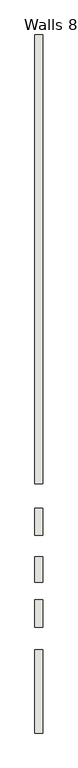
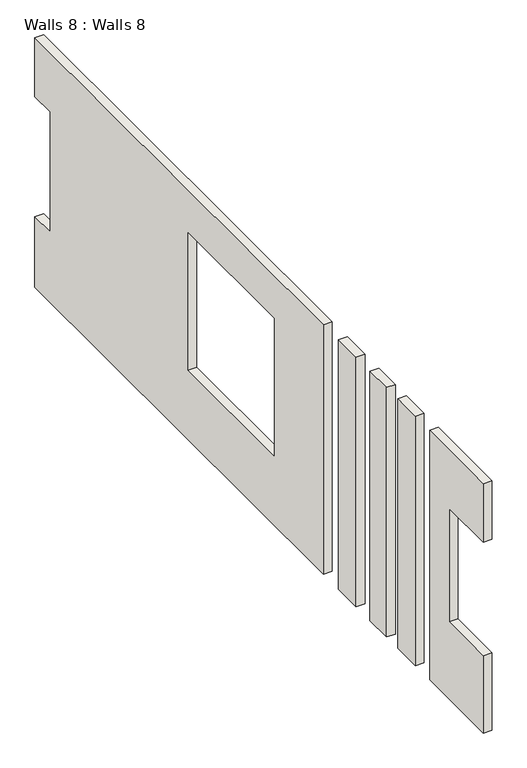
"""IFC4 building model written with IfcOpenShell, lengths in millimetres: wall geometry, Walls 8 : Walls 8."""

from ifc_helpers import new_model, si_unit, frame, origin, place, context, project, spatial, polyline, outline, extrude, source, transform, mapped, element, save


def walls_8_walls_8_57d20523(model_context):
    return source(origin(), model_context, "Body", "SweptSolid", [
        extrude(outline(polyline([(9625.1674246, 17464.824337), (9625.1674246, 15161.2396325), (10106.7589357, 15161.2396325), (10106.7589357, 13807.224337), (1039.9674246, 13807.224337), (1039.9674246, 18592.8), (10106.7589357, 18592.8), (10106.7589357, 17464.824337), (9625.1674246, 17464.824337)]), holes=[polyline([(2589.3674246, 17774.5365374), (2589.3674246, 15135.9493368), (5294.9874401, 15135.9493368), (5294.9874401, 17774.5365374), (2589.3674246, 17774.5365374)])]), frame((-9018.324982, 0.0, 0.0), z_axis=(1.0, 0.0, 0.0), x_axis=(0.0, 1.0, 0.0)), (0.0, 0.0, 1.0), 157.7522082),
        extrude(outline(polyline([(-2922.4325754, 17464.824337), (-3989.2325754, 17464.824337), (-3989.2325754, 18592.8), (-2306.4825754, 18592.8), (-2306.4825754, 13807.224337), (-3989.2325754, 13807.224337), (-3989.2325754, 15294.6370027), (-2922.4325754, 15294.6370027), (-2922.4325754, 17464.824337)])), frame((-9018.324982, 0.0, 0.0), z_axis=(1.0, 0.0, 0.0), x_axis=(0.0, 1.0, 0.0)), (0.0, 0.0, 1.0), 157.7522082),
        extrude(outline(polyline([(-9018.324982, 4.4963312), (-9018.324982, 553.8790064), (-8860.5727738, 553.8790064), (-8860.5727738, 4.4963312), (-9018.324982, 4.4963312)])), frame((0.0, 0.0, 13807.224337), z_axis=(0.0, 0.0, 1.0), x_axis=(1.0, 0.0, 0.0)), (0.0, 0.0, 1.0), 4785.575663),
        extrude(outline(polyline([(-9018.324982, -948.8605015), (-9018.324982, -432.1747353), (-8860.5727738, -432.1747353), (-8860.5727738, -948.8605015), (-9018.324982, -948.8605015)])), frame((0.0, 0.0, 13807.224337), z_axis=(0.0, 0.0, 1.0), x_axis=(1.0, 0.0, 0.0)), (0.0, 0.0, 1.0), 4785.575663),
        extrude(outline(polyline([(-9018.324982, -1855.6325754), (-9018.324982, -1301.807901), (-8860.5727738, -1301.807901), (-8860.5727738, -1855.6325754), (-9018.324982, -1855.6325754)])), frame((0.0, 0.0, 13807.224337), z_axis=(0.0, 0.0, 1.0), x_axis=(1.0, 0.0, 0.0)), (0.0, 0.0, 1.0), 4785.575663),
    ])


if __name__ == "__main__":
    model = new_model("IFC4")
    model_context = context("Model", 3, world=origin())
    ifc_project = project(units=[si_unit("LENGTHUNIT", "METRE", prefix="MILLI")], contexts=[model_context])
    site = spatial("IfcSite", under=ifc_project)
    building = spatial("IfcBuilding", under=site)
    placement = place(None, origin())
    walls_8_walls_8_shape = walls_8_walls_8_57d20523(model_context)
    element("IfcWall", 1, ObjectType="Walls 8 : Walls 8", at=placement, inside=building, context=model_context, shape_type="MappedRepresentation", body=[
        mapped(walls_8_walls_8_shape, transform((0.0, 0.0, 0.0), x_axis=(1.0, 0.0, 0.0), y_axis=(0.0, 1.0, 0.0), z_axis=(0.0, 0.0, 1.0))),
    ])
    save(model, "model.ifc")

# Revit data of these elements
# Element 1 (IfcWall, "Walls 8 : Walls 8")
#   Materials on its faces: "Default Wall"
# Materials
#   "Default Wall": colour RGB 128 128 128, transparency 0
